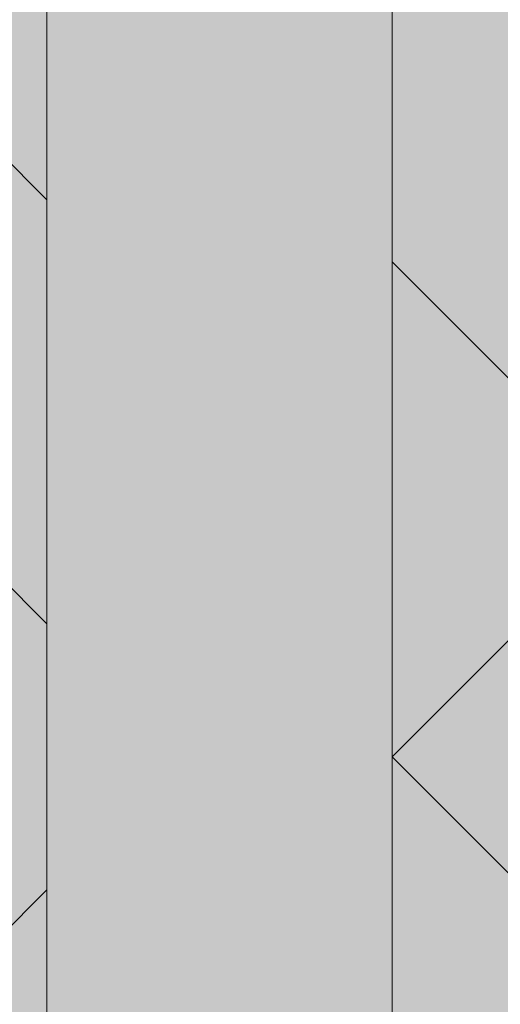
# Model space of a CAD drawing. Units: inches. Extents: x 844 to 2234, y 346 to 1084.
# Tile 35 of 93: x 1261.788 to 1262.676, y 695.763 to 697.583. Entities that reach past the tile are written whole.
import ezdxf

# ---------------------------------------------------------------- set-up
doc = ezdxf.new("R2010")
doc.units = ezdxf.units.IN
doc.header["$MEASUREMENT"] = 0
doc.layers.add('furniture', color=8, linetype='Continuous', lineweight=18)
doc.layers.add('RA-AP-01$0$INT', color=35, linetype='Continuous', lineweight=5)
doc.layers.add('RA-AP-01$0$FURN', color=3, linetype='Continuous')

# ---------------------------------------------------------------- blocks, each defined once
blk = doc.blocks.new('A$C18D01794')
at = {"layer": 'RA-AP-01$0$INT'}
h = blk.add_hatch(color=256, dxfattribs=at)
h.paths.add_polyline_path([(4.46935, -7.07085), (4.50521, -7.035), (4.50521, -7.10671)])
h.paths.add_polyline_path([(4.45521, -7.085), (4.47692, -7.10671), (4.43349, -7.10671)])
h.paths.add_polyline_path([(4.40521, -7.035), (4.44106, -7.07085), (4.40521, -7.10671)])
h.paths.add_polyline_path([(4.42521, -6.91146), (4.45521, -6.88146), (4.48521, -6.91146), (4.48521, -7.02671), (4.45521, -7.05671), (4.42521, -7.02671)])
h.paths.add_polyline_path([(4.50521, -6.83146), (4.50521, -6.90318), (4.46935, -6.86732)])
h.paths.add_polyline_path([(4.42521, -6.70793), (4.45521, -6.67793), (4.48521, -6.70793), (4.48521, -6.82318), (4.45521, -6.85318), (4.42521, -6.82318)])
h.paths.add_polyline_path([(4.42521, -6.50439), (4.45521, -6.47439), (4.48521, -6.50439), (4.48521, -6.61964), (4.45521, -6.64964), (4.42521, -6.61964)])
h.paths.add_polyline_path([(4.46935, -6.66378), (4.50521, -6.62793), (4.50521, -6.69964)])
h.paths.add_polyline_path([(4.40521, -6.62793), (4.44106, -6.66378), (4.40521, -6.69964)])
h.paths.add_polyline_path([(4.40521, -6.42439), (4.44106, -6.46025), (4.40521, -6.49611)])
h.paths.add_polyline_path([(4.46935, -6.46025), (4.50521, -6.42439), (4.50521, -6.49611)])
h.paths.add_polyline_path([(4.42521, -6.30085), (4.45521, -6.27085), (4.48521, -6.30085), (4.48521, -6.41611), (4.45521, -6.44611), (4.42521, -6.41611)])
h.paths.add_polyline_path([(4.42521, -6.22671), (4.47106, -6.22671), (4.42521, -6.27257)])
h.paths.add_polyline_path([(4.49935, -6.22671), (4.63606, -6.22671), (4.66606, -6.25671), (4.63606, -6.28671), (4.49935, -6.28671), (4.46935, -6.25671)])
h.paths.add_polyline_path([(4.68021, -6.27085), (4.71606, -6.30671), (4.64435, -6.30671)])
h.paths.add_polyline_path([(4.64435, -6.20671), (4.71606, -6.20671), (4.68021, -6.24257)])
h.paths.add_polyline_path([(4.72435, -6.22671), (4.86106, -6.22671), (4.89106, -6.25671), (4.86106, -6.28671), (4.72435, -6.28671), (4.69435, -6.25671)])
h.paths.add_polyline_path([(4.90521, -6.27085), (4.94106, -6.30671), (4.86935, -6.30671)])
h.paths.add_polyline_path([(4.86935, -6.20671), (4.94106, -6.20671), (4.90521, -6.24257)])
h.paths.add_polyline_path([(4.94935, -6.22671), (5.08606, -6.22671), (5.11606, -6.25671), (5.08606, -6.28671), (4.94935, -6.28671), (4.91935, -6.25671)])
h.paths.add_polyline_path([(5.13021, -6.27085), (5.16606, -6.30671), (5.09435, -6.30671)])
h.paths.add_polyline_path([(5.09435, -6.20671), (5.16606, -6.20671), (5.13021, -6.24257)])
h.paths.add_polyline_path([(5.17435, -6.22671), (5.31106, -6.22671), (5.34106, -6.25671), (5.31106, -6.28671), (5.17435, -6.28671), (5.14435, -6.25671)])
h.paths.add_polyline_path([(5.32521, -6.30085), (5.35521, -6.27085), (5.38521, -6.30085), (5.38521, -6.41611), (5.35521, -6.44611), (5.32521, -6.41611)])
h.paths.add_polyline_path([(5.33935, -6.22671), (5.38521, -6.22671), (5.38521, -6.27257)])
h.paths.add_polyline_path([(5.32521, -6.50439), (5.35521, -6.47439), (5.38521, -6.50439), (5.38521, -6.61964), (5.35521, -6.64964), (5.32521, -6.61964)])
h.paths.add_polyline_path([(5.30521, -6.42439), (5.34106, -6.46025), (5.30521, -6.49611)])
h.paths.add_polyline_path([(5.36935, -6.46025), (5.40521, -6.42439), (5.40521, -6.49611)])
h.paths.add_polyline_path([(5.40521, -6.62793), (5.40521, -6.69964), (5.36935, -6.66378)])
h.paths.add_polyline_path([(5.30521, -6.62793), (5.34106, -6.66378), (5.30521, -6.69964)])
h.paths.add_polyline_path([(5.32521, -6.70793), (5.35521, -6.67793), (5.38521, -6.70793), (5.38521, -6.82318), (5.35521, -6.85318), (5.32521, -6.82318)])
h.paths.add_polyline_path([(5.30521, -6.83146), (5.34106, -6.86732), (5.30521, -6.90318)])
h.paths.add_polyline_path([(5.32521, -6.91146), (5.35521, -6.88146), (5.38521, -6.91146), (5.38521, -7.02671), (5.35521, -7.05671), (5.32521, -7.02671)])
h.paths.add_polyline_path([(5.40458, -6.83209, 0.001218), (5.40521, -6.83231), (5.40521, -6.90318), (5.36935, -6.86732)])
h.paths.add_polyline_path([(5.36935, -7.07085), (5.40521, -7.035), (5.40521, -7.10671)])
h.paths.add_polyline_path([(5.35521, -7.085), (5.37692, -7.10671), (5.33349, -7.10671)])
h.paths.add_polyline_path([(5.30521, -7.035), (5.34106, -7.07085), (5.30521, -7.10671)])
h = blk.add_hatch(color=256, dxfattribs=at)
h.paths.add_polyline_path([(4.50521, -6.62793), (4.46935, -6.66378), (4.50521, -6.69964), (4.50521, -6.83146), (4.46935, -6.86732), (4.50521, -6.90318), (4.50521, -7.035), (4.46935, -7.07085), (4.50521, -7.10671), (4.47692, -7.10671), (4.45521, -7.085), (4.43349, -7.10671), (4.40521, -7.10671), (4.44106, -7.07085), (4.40521, -7.035), (4.40521, -6.90318), (4.44106, -6.86732), (4.40521, -6.83146), (4.40521, -6.69964), (4.44106, -6.66378), (4.40521, -6.62793), (4.40521, -6.49611), (4.44106, -6.46025), (4.40521, -6.42439), (4.40521, -6.20671), (4.64435, -6.20671), (4.68021, -6.24257), (4.71606, -6.20671), (4.86935, -6.20671), (4.90521, -6.24257), (4.94106, -6.20671), (5.09435, -6.20671), (5.13021, -6.24257), (5.16606, -6.20671), (5.40521, -6.20671), (5.40521, -6.42439), (5.36935, -6.46025), (5.40521, -6.49611), (5.40521, -6.62793), (5.36935, -6.66378), (5.40521, -6.69964), (5.40521, -6.83146), (5.36935, -6.86732), (5.40521, -6.90318), (5.40521, -7.035), (5.36935, -7.07085), (5.40521, -7.10671), (5.37692, -7.10671), (5.35521, -7.085), (5.33349, -7.10671), (5.30521, -7.10671), (5.34106, -7.07085), (5.30521, -7.035), (5.30521, -6.90318), (5.34106, -6.86732), (5.30521, -6.83146), (5.30521, -6.69964), (5.34106, -6.66378), (5.30521, -6.62793), (5.30521, -6.49611), (5.34106, -6.46025), (5.30521, -6.42439), (5.30521, -6.30671), (5.16606, -6.30671), (5.13021, -6.27085), (5.09435, -6.30671), (4.94106, -6.30671), (4.90521, -6.27085), (4.86935, -6.30671), (4.71606, -6.30671), (4.68021, -6.27085), (4.64435, -6.30671), (4.50521, -6.30671), (4.50521, -6.42439), (4.46935, -6.46025), (4.50521, -6.49611)])
h.paths.add_polyline_path([(4.48521, -6.50439), (4.45521, -6.47439), (4.42521, -6.50439), (4.42521, -6.61964), (4.45521, -6.64964), (4.48521, -6.61964)], flags=16)
h.paths.add_polyline_path([(4.45521, -6.44611), (4.48521, -6.41611), (4.48521, -6.30085), (4.45521, -6.27085), (4.42521, -6.30085), (4.42521, -6.41611)], flags=16)
h.paths.add_polyline_path([(4.45521, -6.67793), (4.42521, -6.70793), (4.42521, -6.82318), (4.45521, -6.85318), (4.48521, -6.82318), (4.48521, -6.70793)], flags=16)
h.paths.add_polyline_path([(4.49935, -6.28671), (4.63606, -6.28671), (4.66606, -6.25671), (4.63606, -6.22671), (4.49935, -6.22671), (4.46935, -6.25671)], flags=16)
h.paths.add_polyline_path([(4.42521, -6.27257), (4.47106, -6.22671), (4.42521, -6.22671)], flags=16)
h.paths.add_polyline_path([(4.45521, -6.88146), (4.42521, -6.91146), (4.42521, -7.02671), (4.45521, -7.05671), (4.48521, -7.02671), (4.48521, -6.91146)], flags=16)
h.paths.add_polyline_path([(4.72435, -6.28671), (4.86106, -6.28671), (4.89106, -6.25671), (4.86106, -6.22671), (4.72435, -6.22671), (4.69435, -6.25671)], flags=16)
h.paths.add_polyline_path([(4.91935, -6.25671), (4.94935, -6.28671), (5.08606, -6.28671), (5.11606, -6.25671), (5.08606, -6.22671), (4.94935, -6.22671)], flags=16)
h.paths.add_polyline_path([(5.14435, -6.25671), (5.17435, -6.28671), (5.31106, -6.28671), (5.34106, -6.25671), (5.31106, -6.22671), (5.17435, -6.22671)], flags=16)
h.paths.add_polyline_path([(5.32521, -6.61964), (5.35521, -6.64964), (5.38521, -6.61964), (5.38521, -6.50439), (5.35521, -6.47439), (5.32521, -6.50439)], flags=16)
h.paths.add_polyline_path([(5.32521, -6.41611), (5.35521, -6.44611), (5.38521, -6.41611), (5.38521, -6.30085), (5.35521, -6.27085), (5.32521, -6.30085)], flags=16)
h.paths.add_polyline_path([(5.32521, -6.70793), (5.32521, -6.82318), (5.35521, -6.85318), (5.38521, -6.82318), (5.38521, -6.70793), (5.35521, -6.67793)], flags=16)
h.paths.add_polyline_path([(5.32521, -6.91146), (5.32521, -7.02671), (5.35521, -7.05671), (5.38521, -7.02671), (5.38521, -6.91146), (5.35521, -6.88146)], flags=16)
h.paths.add_polyline_path([(5.33935, -6.22671), (5.38521, -6.27257), (5.38521, -6.22671)], flags=16)
for points in [[(4.50521, -6.30671), (5.30521, -6.30671), (5.30521, -7.10671), (5.25521, -7.10671), (5.25521, -6.35671), (4.55521, -6.35671), (4.55521, -7.10671), (4.50521, -7.10671)], [(4.50521, -7.90671), (5.30521, -7.90671), (5.30521, -7.10671), (5.25521, -7.10671), (5.25521, -7.85671), (4.55521, -7.85671), (4.55521, -7.10671), (4.50521, -7.10671)]]:
    blk.add_hatch(color=256, dxfattribs=at).paths.add_polyline_path(points)
h = blk.add_hatch(color=256, dxfattribs=at)
h.paths.add_polyline_path([(4.58592, -6.35671), (4.55521, -6.35671), (4.55521, -6.38742), (4.8745, -6.70671), (4.90521, -6.676)])
h.paths.add_polyline_path([(5.25521, -6.38742), (5.25521, -6.35671), (5.2245, -6.35671), (4.90521, -6.676), (4.93592, -6.70671)])
h.paths.add_polyline_path([(4.93592, -6.70671), (4.90521, -6.73742), (5.25521, -7.08742), (5.25521, -7.026)])
h.paths.add_polyline_path([(4.55521, -7.026), (4.55521, -7.08742), (4.90521, -6.73742), (4.8745, -6.70671)])
h = blk.add_hatch(color=256, dxfattribs=at)
h.paths.add_polyline_path([(4.58592, -6.35671), (4.6142, -6.35671), (4.66885, -6.41136), (4.72349, -6.35671), (4.77177, -6.35671), (4.82642, -6.41136), (4.86278, -6.375), (4.8445, -6.35671), (4.86278, -6.35671), (4.90521, -6.39914), (4.94763, -6.35671), (4.96592, -6.35671), (4.94763, -6.375), (4.98399, -6.41136), (5.03864, -6.35671), (5.08692, -6.35671), (5.14157, -6.41136), (5.19621, -6.35671), (5.2245, -6.35671), (4.90521, -6.676)])
h.paths.add_polyline_path([(4.89521, -6.63772), (4.89521, -6.52843), (4.84056, -6.58307)], flags=16)
h.paths.add_polyline_path([(4.91521, -6.63772), (4.96985, -6.58307), (4.91521, -6.52843)], flags=16)
h.paths.add_polyline_path([(4.82642, -6.56893), (4.88106, -6.51429), (4.77177, -6.51429)], flags=16)
h.paths.add_polyline_path([(4.98399, -6.56893), (5.03864, -6.51429), (4.92935, -6.51429)], flags=16)
h.paths.add_polyline_path([(4.88106, -6.49429), (4.82642, -6.43964), (4.77177, -6.49429)], flags=16)
h.paths.add_polyline_path([(4.92935, -6.49429), (5.03864, -6.49429), (4.98399, -6.43964)], flags=16)
h.paths.add_polyline_path([(4.89521, -6.48014), (4.89521, -6.40742), (4.87692, -6.38914), (4.84056, -6.4255)], flags=16)
h.paths.add_polyline_path([(4.91521, -6.48014), (4.96985, -6.4255), (4.93349, -6.38914), (4.91521, -6.40742)], flags=16)
h.paths.add_polyline_path([(4.75763, -6.48014), (4.81228, -6.4255), (4.75763, -6.37085)], flags=16)
h.paths.add_polyline_path([(4.73763, -6.48014), (4.73763, -6.37085), (4.68299, -6.4255)], flags=16)
h.paths.add_polyline_path([(5.05278, -6.48014), (5.05278, -6.37085), (4.99814, -6.4255)], flags=16)
h.paths.add_polyline_path([(5.07278, -6.48014), (5.12742, -6.4255), (5.07278, -6.37085)], flags=16)
h.paths.add_polyline_path([(4.93592, -6.70671), (5.25521, -6.38742), (5.25521, -6.41571), (5.20056, -6.47035), (5.25521, -6.525), (5.25521, -6.57328), (5.20056, -6.62793), (5.23692, -6.66429), (5.25521, -6.646), (5.25521, -6.66429), (5.21278, -6.70671), (5.25521, -6.74914), (5.25521, -6.76742), (5.23692, -6.74914), (5.20056, -6.7855), (5.25521, -6.84014), (5.25521, -6.88843), (5.20056, -6.94307), (5.25521, -6.99772), (5.25521, -7.026)])
h.paths.add_polyline_path([(5.04299, -6.7855), (5.09763, -6.84014), (5.09763, -6.73085)], flags=16)
h.paths.add_polyline_path([(5.02885, -6.77136), (5.08349, -6.71671), (4.9742, -6.71671)], flags=16)
h.paths.add_polyline_path([(5.11763, -6.84014), (5.17228, -6.7855), (5.11763, -6.73085)], flags=16)
h.paths.add_polyline_path([(5.08349, -6.69671), (5.02885, -6.64207), (4.9742, -6.69671)], flags=16)
h.paths.add_polyline_path([(5.13177, -6.85429), (5.18642, -6.79964), (5.24106, -6.85429)], flags=17)
h.paths.add_polyline_path([(5.13177, -6.71671), (5.18642, -6.77136), (5.22278, -6.735), (5.2045, -6.71671)], flags=16)
h.paths.add_polyline_path([(5.09763, -6.68257), (5.09763, -6.57328), (5.04299, -6.62793)], flags=16)
h.paths.add_polyline_path([(5.13177, -6.87429), (5.24106, -6.87429), (5.18642, -6.92893)], flags=17)
h.paths.add_polyline_path([(5.13177, -6.69671), (5.2045, -6.69671), (5.22278, -6.67843), (5.18642, -6.64207)], flags=16)
h.paths.add_polyline_path([(5.11763, -6.68257), (5.17228, -6.62793), (5.11763, -6.57328)], flags=16)
h.paths.add_polyline_path([(5.18642, -6.61378), (5.24106, -6.55914), (5.13177, -6.55914)], flags=16)
h.paths.add_polyline_path([(5.13177, -6.53914), (5.24106, -6.53914), (5.18642, -6.48449)], flags=16)
h.paths.add_polyline_path([(5.25521, -7.08742), (5.25521, -7.10671), (4.55521, -7.10671), (4.55521, -7.08742), (4.90521, -6.73742)])
h.paths.add_polyline_path([(4.98399, -6.84449), (4.92935, -6.89914), (5.03864, -6.89914)], flags=16)
h.paths.add_polyline_path([(4.96985, -6.83035), (4.91521, -6.77571), (4.91521, -6.885)], flags=16)
h.paths.add_polyline_path([(4.92935, -6.91914), (4.98399, -6.97378), (5.03864, -6.91914)], flags=16)
h.paths.add_polyline_path([(5.05278, -6.93328), (4.99814, -6.98793), (5.05278, -7.04257)], flags=16)
h.paths.add_polyline_path([(5.07278, -6.93328), (5.07278, -7.04257), (5.12742, -6.98793)], flags=16)
h.paths.add_polyline_path([(4.89521, -6.77571), (4.84056, -6.83035), (4.89521, -6.885)], flags=16)
h.paths.add_polyline_path([(4.91521, -6.93328), (4.91521, -7.006), (4.93349, -7.02429), (4.96985, -6.98793)], flags=16)
h.paths.add_polyline_path([(4.88106, -6.89914), (4.82642, -6.84449), (4.77177, -6.89914)], flags=16)
h.paths.add_polyline_path([(4.89521, -6.93328), (4.84056, -6.98793), (4.87692, -7.02429), (4.89521, -7.006)], flags=16)
h.paths.add_polyline_path([(4.98399, -7.00207), (4.94763, -7.03843), (4.96592, -7.05671), (5.03864, -7.05671)], flags=16)
h.paths.add_polyline_path([(4.88106, -6.91914), (4.77177, -6.91914), (4.82642, -6.97378)], flags=16)
h.paths.add_polyline_path([(4.90521, -7.01429), (4.86278, -7.05671), (4.94763, -7.05671)], flags=16)
h.paths.add_polyline_path([(5.14157, -7.00207), (5.08692, -7.05671), (5.19621, -7.05671)], flags=16)
h.paths.add_polyline_path([(4.82642, -7.00207), (4.77177, -7.05671), (4.8445, -7.05671), (4.86278, -7.03843)], flags=16)
h.paths.add_polyline_path([(4.81228, -6.98793), (4.75763, -6.93328), (4.75763, -7.04257)], flags=16)
h.paths.add_polyline_path([(4.73763, -6.93328), (4.68299, -6.98793), (4.73763, -7.04257)], flags=16)
h.paths.add_polyline_path([(4.72349, -7.05671), (4.66885, -7.00207), (4.6142, -7.05671)], flags=16)
h.paths.add_polyline_path([(4.59763, -6.70671), (4.55521, -6.66429), (4.55521, -6.646), (4.57349, -6.66429), (4.60985, -6.62793), (4.55521, -6.57328), (4.55521, -6.525), (4.60985, -6.47035), (4.55521, -6.41571), (4.55521, -6.38742), (4.8745, -6.70671), (4.55521, -7.026), (4.55521, -6.99772), (4.60985, -6.94307), (4.55521, -6.88843), (4.55521, -6.84014), (4.60985, -6.7855), (4.57349, -6.74914), (4.55521, -6.76742), (4.55521, -6.74914)])
h.paths.add_polyline_path([(4.71278, -6.73085), (4.71278, -6.84014), (4.76742, -6.7855)], flags=16)
h.paths.add_polyline_path([(4.72692, -6.71671), (4.78157, -6.77136), (4.83621, -6.71671)], flags=16)
h.paths.add_polyline_path([(4.69278, -6.73085), (4.63814, -6.7855), (4.69278, -6.84014)], flags=16)
h.paths.add_polyline_path([(4.72692, -6.69671), (4.83621, -6.69671), (4.78157, -6.64207)], flags=16)
h.paths.add_polyline_path([(4.67864, -6.71671), (4.60592, -6.71671), (4.58763, -6.735), (4.62399, -6.77136)], flags=16)
h.paths.add_polyline_path([(4.71278, -6.68257), (4.76742, -6.62793), (4.71278, -6.57328)], flags=16)
h.paths.add_polyline_path([(4.67864, -6.69671), (4.62399, -6.64207), (4.58763, -6.67843), (4.60592, -6.69671)], flags=16)
h.paths.add_polyline_path([(4.69278, -6.68257), (4.69278, -6.57328), (4.63814, -6.62793)], flags=16)
h.paths.add_polyline_path([(4.62399, -6.79964), (4.67864, -6.85429), (4.56935, -6.85429)], flags=17)
h.paths.add_polyline_path([(4.62399, -6.61378), (4.67864, -6.55914), (4.56935, -6.55914)], flags=16)
h.paths.add_polyline_path([(4.67864, -6.87429), (4.62399, -6.92893), (4.56935, -6.87429)], flags=17)
h.paths.add_polyline_path([(4.67864, -6.53914), (4.62399, -6.48449), (4.56935, -6.53914)], flags=16)
h = blk.add_hatch(color=256, dxfattribs=at)
h.paths.add_polyline_path([(4.50521, -7.5855), (4.46935, -7.54964), (4.50521, -7.51378), (4.50521, -7.38196), (4.46935, -7.34611), (4.50521, -7.31025), (4.50521, -7.17843), (4.46935, -7.14257), (4.50521, -7.10671), (4.47692, -7.10671), (4.45521, -7.12843), (4.43349, -7.10671), (4.40521, -7.10671), (4.44106, -7.14257), (4.40521, -7.17843), (4.40521, -7.31025), (4.44106, -7.34611), (4.40521, -7.38196), (4.40521, -7.51378), (4.44106, -7.54964), (4.40521, -7.5855), (4.40521, -7.71732), (4.44106, -7.75318), (4.40521, -7.78903), (4.40521, -8.00671), (4.64435, -8.00671), (4.68021, -7.97085), (4.71606, -8.00671), (4.86935, -8.00671), (4.90521, -7.97085), (4.94106, -8.00671), (5.09435, -8.00671), (5.13021, -7.97085), (5.16606, -8.00671), (5.40521, -8.00671), (5.40521, -7.78903), (5.36935, -7.75318), (5.40521, -7.71732), (5.40521, -7.5855), (5.36935, -7.54964), (5.40521, -7.51378), (5.40521, -7.38196), (5.36935, -7.34611), (5.40521, -7.31025), (5.40521, -7.17843), (5.36935, -7.14257), (5.40521, -7.10671), (5.37692, -7.10671), (5.35521, -7.12843), (5.33349, -7.10671), (5.30521, -7.10671), (5.34106, -7.14257), (5.30521, -7.17843), (5.30521, -7.31025), (5.34106, -7.34611), (5.30521, -7.38196), (5.30521, -7.51378), (5.34106, -7.54964), (5.30521, -7.5855), (5.30521, -7.71732), (5.34106, -7.75318), (5.30521, -7.78903), (5.30521, -7.90671), (5.16606, -7.90671), (5.13021, -7.94257), (5.09435, -7.90671), (4.94106, -7.90671), (4.90521, -7.94257), (4.86935, -7.90671), (4.71606, -7.90671), (4.68021, -7.94257), (4.64435, -7.90671), (4.50521, -7.90671), (4.50521, -7.78903), (4.46935, -7.75318), (4.50521, -7.71732)])
h.paths.add_polyline_path([(4.48521, -7.70903), (4.45521, -7.73903), (4.42521, -7.70903), (4.42521, -7.59378), (4.45521, -7.56378), (4.48521, -7.59378)], flags=16)
h.paths.add_polyline_path([(4.45521, -7.76732), (4.48521, -7.79732), (4.48521, -7.91257), (4.45521, -7.94257), (4.42521, -7.91257), (4.42521, -7.79732)], flags=16)
h.paths.add_polyline_path([(4.45521, -7.5355), (4.42521, -7.5055), (4.42521, -7.39025), (4.45521, -7.36025), (4.48521, -7.39025), (4.48521, -7.5055)], flags=16)
h.paths.add_polyline_path([(4.49935, -7.92671), (4.63606, -7.92671), (4.66606, -7.95671), (4.63606, -7.98671), (4.49935, -7.98671), (4.46935, -7.95671)], flags=16)
h.paths.add_polyline_path([(4.42521, -7.94085), (4.47106, -7.98671), (4.42521, -7.98671)], flags=16)
h.paths.add_polyline_path([(4.45521, -7.33196), (4.42521, -7.30196), (4.42521, -7.18671), (4.45521, -7.15671), (4.48521, -7.18671), (4.48521, -7.30196)], flags=16)
h.paths.add_polyline_path([(4.72435, -7.92671), (4.86106, -7.92671), (4.89106, -7.95671), (4.86106, -7.98671), (4.72435, -7.98671), (4.69435, -7.95671)], flags=16)
h.paths.add_polyline_path([(4.91935, -7.95671), (4.94935, -7.92671), (5.08606, -7.92671), (5.11606, -7.95671), (5.08606, -7.98671), (4.94935, -7.98671)], flags=16)
h.paths.add_polyline_path([(5.14435, -7.95671), (5.17435, -7.92671), (5.31106, -7.92671), (5.34106, -7.95671), (5.31106, -7.98671), (5.17435, -7.98671)], flags=16)
h.paths.add_polyline_path([(5.32521, -7.59378), (5.35521, -7.56378), (5.38521, -7.59378), (5.38521, -7.70903), (5.35521, -7.73903), (5.32521, -7.70903)], flags=16)
h.paths.add_polyline_path([(5.32521, -7.79732), (5.35521, -7.76732), (5.38521, -7.79732), (5.38521, -7.91257), (5.35521, -7.94257), (5.32521, -7.91257)], flags=16)
h.paths.add_polyline_path([(5.32521, -7.5055), (5.32521, -7.39025), (5.35521, -7.36025), (5.38521, -7.39025), (5.38521, -7.5055), (5.35521, -7.5355)], flags=16)
h.paths.add_polyline_path([(5.32521, -7.30196), (5.32521, -7.18671), (5.35521, -7.15671), (5.38521, -7.18671), (5.38521, -7.30196), (5.35521, -7.33196)], flags=16)
h.paths.add_polyline_path([(5.33935, -7.98671), (5.38521, -7.94085), (5.38521, -7.98671)], flags=16)
h = blk.add_hatch(color=256, dxfattribs=at)
h.paths.add_polyline_path([(4.46935, -7.14257), (4.50521, -7.17843), (4.50521, -7.10671)])
h.paths.add_polyline_path([(4.45521, -7.12843), (4.47692, -7.10671), (4.43349, -7.10671)])
h.paths.add_polyline_path([(4.40521, -7.17843), (4.44106, -7.14257), (4.40521, -7.10671)])
h.paths.add_polyline_path([(4.42521, -7.30196), (4.45521, -7.33196), (4.48521, -7.30196), (4.48521, -7.18671), (4.45521, -7.15671), (4.42521, -7.18671)])
h.paths.add_polyline_path([(4.50521, -7.38196), (4.50521, -7.31025), (4.46935, -7.34611)])
h.paths.add_polyline_path([(4.42521, -7.5055), (4.45521, -7.5355), (4.48521, -7.5055), (4.48521, -7.39025), (4.45521, -7.36025), (4.42521, -7.39025)])
h.paths.add_polyline_path([(4.42521, -7.70903), (4.45521, -7.73903), (4.48521, -7.70903), (4.48521, -7.59378), (4.45521, -7.56378), (4.42521, -7.59378)])
h.paths.add_polyline_path([(4.46935, -7.54964), (4.50521, -7.5855), (4.50521, -7.51378)])
h.paths.add_polyline_path([(4.40521, -7.5855), (4.44106, -7.54964), (4.40521, -7.51378)])
h.paths.add_polyline_path([(4.40521, -7.78903), (4.44106, -7.75318), (4.40521, -7.71732)])
h.paths.add_polyline_path([(4.46935, -7.75318), (4.50521, -7.78903), (4.50521, -7.71732)])
h.paths.add_polyline_path([(4.42521, -7.91257), (4.45521, -7.94257), (4.48521, -7.91257), (4.48521, -7.79732), (4.45521, -7.76732), (4.42521, -7.79732)])
h.paths.add_polyline_path([(4.42521, -7.98671), (4.47106, -7.98671), (4.42521, -7.94085)])
h.paths.add_polyline_path([(4.49935, -7.98671), (4.63606, -7.98671), (4.66606, -7.95671), (4.63606, -7.92671), (4.49935, -7.92671), (4.46935, -7.95671)])
h.paths.add_polyline_path([(4.68021, -7.94257), (4.71606, -7.90671), (4.64435, -7.90671)])
h.paths.add_polyline_path([(4.64435, -8.00671), (4.71606, -8.00671), (4.68021, -7.97085)])
h.paths.add_polyline_path([(4.72435, -7.98671), (4.86106, -7.98671), (4.89106, -7.95671), (4.86106, -7.92671), (4.72435, -7.92671), (4.69435, -7.95671)])
h.paths.add_polyline_path([(4.90521, -7.94257), (4.94106, -7.90671), (4.86935, -7.90671)])
h.paths.add_polyline_path([(4.86935, -8.00671), (4.94106, -8.00671), (4.90521, -7.97085)])
h.paths.add_polyline_path([(4.94935, -7.98671), (5.08606, -7.98671), (5.11606, -7.95671), (5.08606, -7.92671), (4.94935, -7.92671), (4.91935, -7.95671)])
h.paths.add_polyline_path([(5.13021, -7.94257), (5.16606, -7.90671), (5.09435, -7.90671)])
h.paths.add_polyline_path([(5.09435, -8.00671), (5.16606, -8.00671), (5.13021, -7.97085)])
h.paths.add_polyline_path([(5.17435, -7.98671), (5.31106, -7.98671), (5.34106, -7.95671), (5.31106, -7.92671), (5.17435, -7.92671), (5.14435, -7.95671)])
h.paths.add_polyline_path([(5.32521, -7.91257), (5.35521, -7.94257), (5.38521, -7.91257), (5.38521, -7.79732), (5.35521, -7.76732), (5.32521, -7.79732)])
h.paths.add_polyline_path([(5.33935, -7.98671), (5.38521, -7.98671), (5.38521, -7.94085)])
h.paths.add_polyline_path([(5.32521, -7.70903), (5.35521, -7.73903), (5.38521, -7.70903), (5.38521, -7.59378), (5.35521, -7.56378), (5.32521, -7.59378)])
h.paths.add_polyline_path([(5.30521, -7.78903), (5.34106, -7.75318), (5.30521, -7.71732)])
h.paths.add_polyline_path([(5.36935, -7.75318), (5.40521, -7.78903), (5.40521, -7.71732)])
h.paths.add_polyline_path([(5.40521, -7.5855), (5.40521, -7.51378), (5.36935, -7.54964)])
h.paths.add_polyline_path([(5.30521, -7.5855), (5.34106, -7.54964), (5.30521, -7.51378)])
h.paths.add_polyline_path([(5.32521, -7.5055), (5.35521, -7.5355), (5.38521, -7.5055), (5.38521, -7.39025), (5.35521, -7.36025), (5.32521, -7.39025)])
h.paths.add_polyline_path([(5.30521, -7.38196), (5.34106, -7.34611), (5.30521, -7.31025)])
h.paths.add_polyline_path([(5.32521, -7.30196), (5.35521, -7.33196), (5.38521, -7.30196), (5.38521, -7.18671), (5.35521, -7.15671), (5.32521, -7.18671)])
h.paths.add_polyline_path([(5.40458, -7.38134, -0.001218), (5.40521, -7.38111), (5.40521, -7.31025), (5.36935, -7.34611)])
h.paths.add_polyline_path([(5.36935, -7.14257), (5.40521, -7.17843), (5.40521, -7.10671)])
h.paths.add_polyline_path([(5.35521, -7.12843), (5.37692, -7.10671), (5.33349, -7.10671)])
h.paths.add_polyline_path([(5.30521, -7.17843), (5.34106, -7.14257), (5.30521, -7.10671)])
h = blk.add_hatch(color=256, dxfattribs=at)
h.paths.add_polyline_path([(4.58592, -7.85671), (4.6142, -7.85671), (4.66885, -7.80207), (4.72349, -7.85671), (4.77177, -7.85671), (4.82642, -7.80207), (4.86278, -7.83843), (4.8445, -7.85671), (4.86278, -7.85671), (4.90521, -7.81429), (4.94763, -7.85671), (4.96592, -7.85671), (4.94763, -7.83843), (4.98399, -7.80207), (5.03864, -7.85671), (5.08692, -7.85671), (5.14157, -7.80207), (5.19621, -7.85671), (5.2245, -7.85671), (4.90521, -7.53742)])
h.paths.add_polyline_path([(4.89521, -7.57571), (4.89521, -7.685), (4.84056, -7.63035)], flags=16)
h.paths.add_polyline_path([(4.91521, -7.57571), (4.96985, -7.63035), (4.91521, -7.685)], flags=16)
h.paths.add_polyline_path([(4.82642, -7.64449), (4.88106, -7.69914), (4.77177, -7.69914)], flags=16)
h.paths.add_polyline_path([(4.98399, -7.64449), (5.03864, -7.69914), (4.92935, -7.69914)], flags=16)
h.paths.add_polyline_path([(4.88106, -7.71914), (4.82642, -7.77378), (4.77177, -7.71914)], flags=16)
h.paths.add_polyline_path([(4.92935, -7.71914), (5.03864, -7.71914), (4.98399, -7.77378)], flags=16)
h.paths.add_polyline_path([(4.89521, -7.73328), (4.89521, -7.806), (4.87692, -7.82429), (4.84056, -7.78793)], flags=16)
h.paths.add_polyline_path([(4.91521, -7.73328), (4.96985, -7.78793), (4.93349, -7.82429), (4.91521, -7.806)], flags=16)
h.paths.add_polyline_path([(4.75763, -7.73328), (4.81228, -7.78793), (4.75763, -7.84257)], flags=16)
h.paths.add_polyline_path([(4.73763, -7.73328), (4.73763, -7.84257), (4.68299, -7.78793)], flags=16)
h.paths.add_polyline_path([(5.05278, -7.73328), (5.05278, -7.84257), (4.99814, -7.78793)], flags=16)
h.paths.add_polyline_path([(5.07278, -7.73328), (5.12742, -7.78793), (5.07278, -7.84257)], flags=16)
h.paths.add_polyline_path([(4.93592, -7.50671), (5.25521, -7.826), (5.25521, -7.79772), (5.20056, -7.74307), (5.25521, -7.68843), (5.25521, -7.64014), (5.20056, -7.5855), (5.23692, -7.54914), (5.25521, -7.56742), (5.25521, -7.54914), (5.21278, -7.50671), (5.25521, -7.46429), (5.25521, -7.446), (5.23692, -7.46429), (5.20056, -7.42793), (5.25521, -7.37328), (5.25521, -7.325), (5.20056, -7.27035), (5.25521, -7.21571), (5.25521, -7.18742)])
h.paths.add_polyline_path([(5.04299, -7.42793), (5.09763, -7.37328), (5.09763, -7.48257)], flags=16)
h.paths.add_polyline_path([(5.02885, -7.44207), (5.08349, -7.49671), (4.9742, -7.49671)], flags=16)
h.paths.add_polyline_path([(5.11763, -7.37328), (5.17228, -7.42793), (5.11763, -7.48257)], flags=16)
h.paths.add_polyline_path([(5.08349, -7.51671), (5.02885, -7.57136), (4.9742, -7.51671)], flags=16)
h.paths.add_polyline_path([(5.13177, -7.35914), (5.18642, -7.41378), (5.24106, -7.35914)], flags=17)
h.paths.add_polyline_path([(5.13177, -7.49671), (5.18642, -7.44207), (5.22278, -7.47843), (5.2045, -7.49671)], flags=16)
h.paths.add_polyline_path([(5.09763, -7.53085), (5.09763, -7.64014), (5.04299, -7.5855)], flags=16)
h.paths.add_polyline_path([(5.13177, -7.33914), (5.24106, -7.33914), (5.18642, -7.28449)], flags=17)
h.paths.add_polyline_path([(5.13177, -7.51671), (5.2045, -7.51671), (5.22278, -7.535), (5.18642, -7.57136)], flags=16)
h.paths.add_polyline_path([(5.11763, -7.53085), (5.17228, -7.5855), (5.11763, -7.64014)], flags=16)
h.paths.add_polyline_path([(5.18642, -7.59964), (5.24106, -7.65429), (5.13177, -7.65429)], flags=16)
h.paths.add_polyline_path([(5.13177, -7.67429), (5.24106, -7.67429), (5.18642, -7.72893)], flags=16)
h.paths.add_polyline_path([(5.25521, -7.126), (5.25521, -7.10671), (4.55521, -7.10671), (4.55521, -7.126), (4.90521, -7.476)])
h.paths.add_polyline_path([(4.98399, -7.36893), (4.92935, -7.31429), (5.03864, -7.31429)], flags=16)
h.paths.add_polyline_path([(4.96985, -7.38307), (4.91521, -7.43772), (4.91521, -7.32843)], flags=16)
h.paths.add_polyline_path([(4.92935, -7.29429), (4.98399, -7.23964), (5.03864, -7.29429)], flags=16)
h.paths.add_polyline_path([(5.05278, -7.28014), (4.99814, -7.2255), (5.05278, -7.17085)], flags=16)
h.paths.add_polyline_path([(5.07278, -7.28014), (5.07278, -7.17085), (5.12742, -7.2255)], flags=16)
h.paths.add_polyline_path([(4.89521, -7.43772), (4.84056, -7.38307), (4.89521, -7.32843)], flags=16)
h.paths.add_polyline_path([(4.91521, -7.28014), (4.91521, -7.20742), (4.93349, -7.18914), (4.96985, -7.2255)], flags=16)
h.paths.add_polyline_path([(4.88106, -7.31429), (4.82642, -7.36893), (4.77177, -7.31429)], flags=16)
h.paths.add_polyline_path([(4.89521, -7.28014), (4.84056, -7.2255), (4.87692, -7.18914), (4.89521, -7.20742)], flags=16)
h.paths.add_polyline_path([(4.98399, -7.21136), (4.94763, -7.175), (4.96592, -7.15671), (5.03864, -7.15671)], flags=16)
h.paths.add_polyline_path([(4.88106, -7.29429), (4.77177, -7.29429), (4.82642, -7.23964)], flags=16)
h.paths.add_polyline_path([(4.90521, -7.19914), (4.86278, -7.15671), (4.94763, -7.15671)], flags=16)
h.paths.add_polyline_path([(5.14157, -7.21136), (5.08692, -7.15671), (5.19621, -7.15671)], flags=16)
h.paths.add_polyline_path([(4.82642, -7.21136), (4.77177, -7.15671), (4.8445, -7.15671), (4.86278, -7.175)], flags=16)
h.paths.add_polyline_path([(4.81228, -7.2255), (4.75763, -7.28014), (4.75763, -7.17085)], flags=16)
h.paths.add_polyline_path([(4.73763, -7.28014), (4.68299, -7.2255), (4.73763, -7.17085)], flags=16)
h.paths.add_polyline_path([(4.72349, -7.15671), (4.66885, -7.21136), (4.6142, -7.15671)], flags=16)
h.paths.add_polyline_path([(4.59763, -7.50671), (4.55521, -7.54914), (4.55521, -7.56742), (4.57349, -7.54914), (4.60985, -7.5855), (4.55521, -7.64014), (4.55521, -7.68843), (4.60985, -7.74307), (4.55521, -7.79772), (4.55521, -7.826), (4.8745, -7.50671), (4.55521, -7.18742), (4.55521, -7.21571), (4.60985, -7.27035), (4.55521, -7.325), (4.55521, -7.37328), (4.60985, -7.42793), (4.57349, -7.46429), (4.55521, -7.446), (4.55521, -7.46429)])
h.paths.add_polyline_path([(4.71278, -7.48257), (4.71278, -7.37328), (4.76742, -7.42793)], flags=16)
h.paths.add_polyline_path([(4.72692, -7.49671), (4.78157, -7.44207), (4.83621, -7.49671)], flags=16)
h.paths.add_polyline_path([(4.69278, -7.48257), (4.63814, -7.42793), (4.69278, -7.37328)], flags=16)
h.paths.add_polyline_path([(4.72692, -7.51671), (4.83621, -7.51671), (4.78157, -7.57136)], flags=16)
h.paths.add_polyline_path([(4.67864, -7.49671), (4.60592, -7.49671), (4.58763, -7.47843), (4.62399, -7.44207)], flags=16)
h.paths.add_polyline_path([(4.71278, -7.53085), (4.76742, -7.5855), (4.71278, -7.64014)], flags=16)
h.paths.add_polyline_path([(4.67864, -7.51671), (4.62399, -7.57136), (4.58763, -7.535), (4.60592, -7.51671)], flags=16)
h.paths.add_polyline_path([(4.69278, -7.53085), (4.69278, -7.64014), (4.63814, -7.5855)], flags=16)
h.paths.add_polyline_path([(4.62399, -7.41378), (4.67864, -7.35914), (4.56935, -7.35914)], flags=17)
h.paths.add_polyline_path([(4.62399, -7.59964), (4.67864, -7.65429), (4.56935, -7.65429)], flags=16)
h.paths.add_polyline_path([(4.67864, -7.33914), (4.62399, -7.28449), (4.56935, -7.33914)], flags=17)
h.paths.add_polyline_path([(4.67864, -7.67429), (4.62399, -7.72893), (4.56935, -7.67429)], flags=16)
h = blk.add_hatch(color=256, dxfattribs=at)
h.paths.add_polyline_path([(4.90521, -7.53742), (4.8745, -7.50671), (4.55521, -7.826), (4.55521, -7.85671), (4.58592, -7.85671)])
h.paths.add_polyline_path([(4.93592, -7.50671), (4.90521, -7.53742), (5.2245, -7.85671), (5.25521, -7.85671), (5.25521, -7.826)])
h.paths.add_polyline_path([(5.25521, -7.18742), (5.25521, -7.126), (4.90521, -7.476), (4.93592, -7.50671)])
h.paths.add_polyline_path([(4.8745, -7.50671), (4.90521, -7.476), (4.55521, -7.126), (4.55521, -7.18742)])
for p, q in [((4.55521, -7.10671), (4.55521, -6.35671)), ((4.90521, -6.73742), (4.55521, -7.08742)), ((4.46935, -7.07085), (4.50521, -7.10671)), ((4.46935, -7.14257), (4.50521, -7.10671)), ((4.55521, -7.10671), (4.55521, -7.85671)), ((4.90521, -7.476), (4.55521, -7.126)), ((4.50521, -7.17843), (4.46935, -7.14257)), ((4.8745, -7.50671), (4.55521, -7.18742))]:
    blk.add_line(p, q, dxfattribs=at)
for points in [[(5.30521, -7.10671), (5.30521, -6.30671), (4.50521, -6.30671), (4.50521, -7.10671)], [(5.30521, -7.10671), (5.30521, -7.90671), (4.50521, -7.90671), (4.50521, -7.10671)]]:
    blk.add_lwpolyline(points, dxfattribs=at)
blk = doc.blocks.new('A$C5D2F253E')
at = {"layer": 'RA-AP-01$0$FURN', "xscale": -0.7999999999883585, "yscale": 0.7999999999883585, "zscale": 0.8, "rotation": 90}
blk.add_blockref('A$C18D01794', (-5.68776, 4.75792), dxfattribs=at)

msp = doc.modelspace()

# ---------------------------------------------------------------- block references
at = {"layer": 'furniture', "xscale": -15.94108302203742, "yscale": 15.94108302203742, "zscale": 15.94108302203742, "rotation": 270}
msp.add_blockref('A$C5D2F253E', (1244.0841, 696.2585), dxfattribs=at)

doc.saveas('drawing.dxf')
